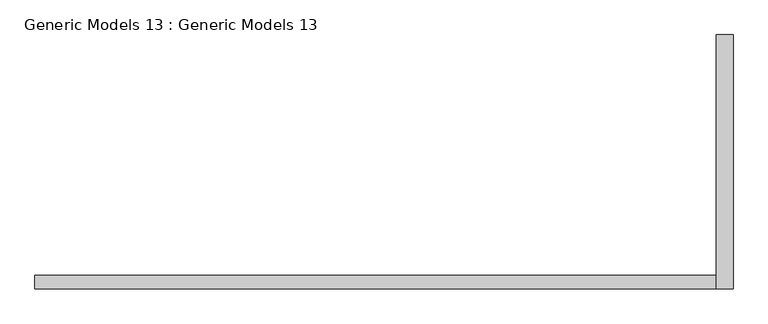
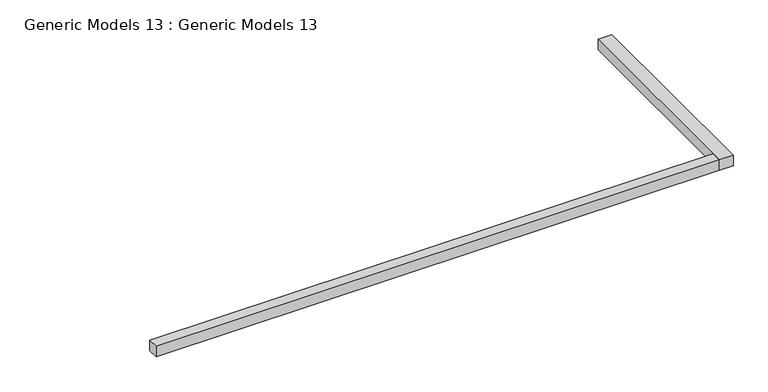
"""IFC4 building model written with IfcOpenShell, lengths in millimetres: proxy geometry, Generic Models 13 : Generic Models 13."""

from ifc_helpers import new_model, si_unit, frame, origin, place, context, project, spatial, polyline, outline, extrude, source, transform, mapped, element, save


def generic_models_13_generic_models_13_04127036(model_context):
    return source(origin(), model_context, "Body", "SweptSolid", [
        extrude(outline(polyline([(-12235.5371373, -3487.8992555), (-12299.0371373, -3487.8992555), (-12299.0371373, -2516.661407), (-12235.5371373, -2516.661407), (-12235.5371373, -3487.8992555)])), frame((0.0, 0.0, 4521.3498465), z_axis=(0.0, 0.0, 1.0), x_axis=(1.0, 0.0, 0.0)), (0.0, 0.0, 1.0), 50.8),
        extrude(outline(polyline([(-12299.0371373, -3437.0992555), (-12299.0371373, -3487.8992555), (-14902.5371373, -3487.8992555), (-14902.5371373, -3437.0992555), (-12299.0371373, -3437.0992555)])), frame((0.0, 0.0, 4521.3498465), z_axis=(0.0, 0.0, 1.0), x_axis=(1.0, 0.0, 0.0)), (0.0, 0.0, 1.0), 50.8),
    ])


if __name__ == "__main__":
    model = new_model("IFC4")
    model_context = context("Model", 3, world=origin())
    ifc_project = project(units=[si_unit("LENGTHUNIT", "METRE", prefix="MILLI")], contexts=[model_context])
    site = spatial("IfcSite", under=ifc_project)
    building = spatial("IfcBuilding", under=site)
    placement = place(None, origin())
    generic_models_13_generic_models_13_shape = generic_models_13_generic_models_13_04127036(model_context)
    element("IfcBuildingElementProxy", 1, Name="Generic Models 13 : Generic Models 13", ObjectType="Generic Models 13 : Generic Models 13", at=placement, inside=building, context=model_context, shape_type="MappedRepresentation", body=[
        mapped(generic_models_13_generic_models_13_shape, transform((0.0, 0.0, 0.0), x_axis=(1.0, 0.0, 0.0), y_axis=(0.0, 1.0, 0.0), z_axis=(0.0, 0.0, 1.0))),
    ])
    save(model, "model.ifc")

# Revit data of these elements
# Element 1 (IfcBuildingElementProxy, "Generic Models 13 : Generic Models 13")
#   Materials on its faces: "Steel, Carbon", "Steel, Chrome Plated"
# Materials
#   "Steel, Carbon": class "Metal", colour RGB 0 0 0, transparency 0, Description = "Carbon steel", Cost = 0
#   "Steel, Chrome Plated": class "Metal", colour RGB 17 17 17, transparency 0, Description = "Chromiuim plated steel", Cost = 0
